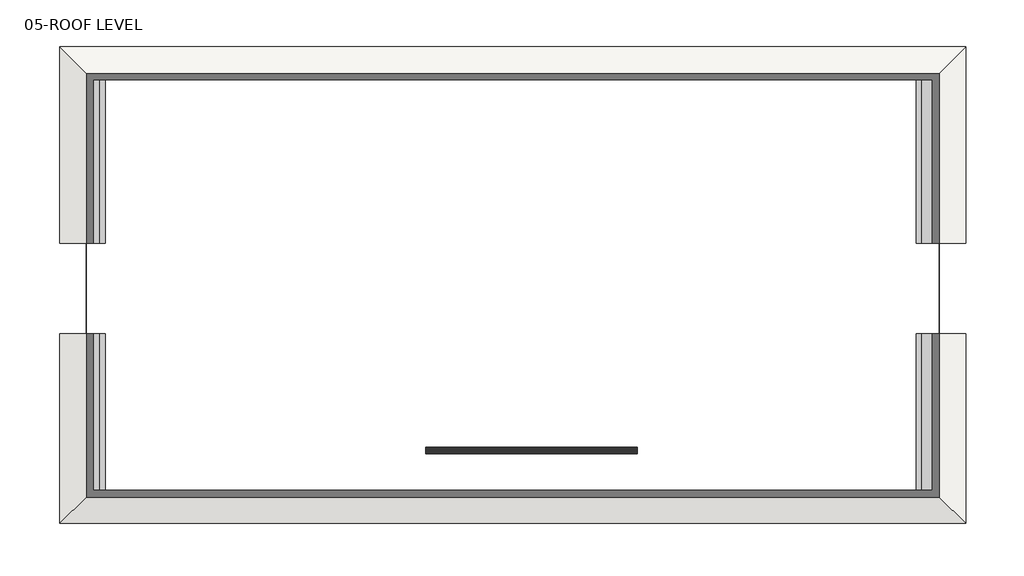
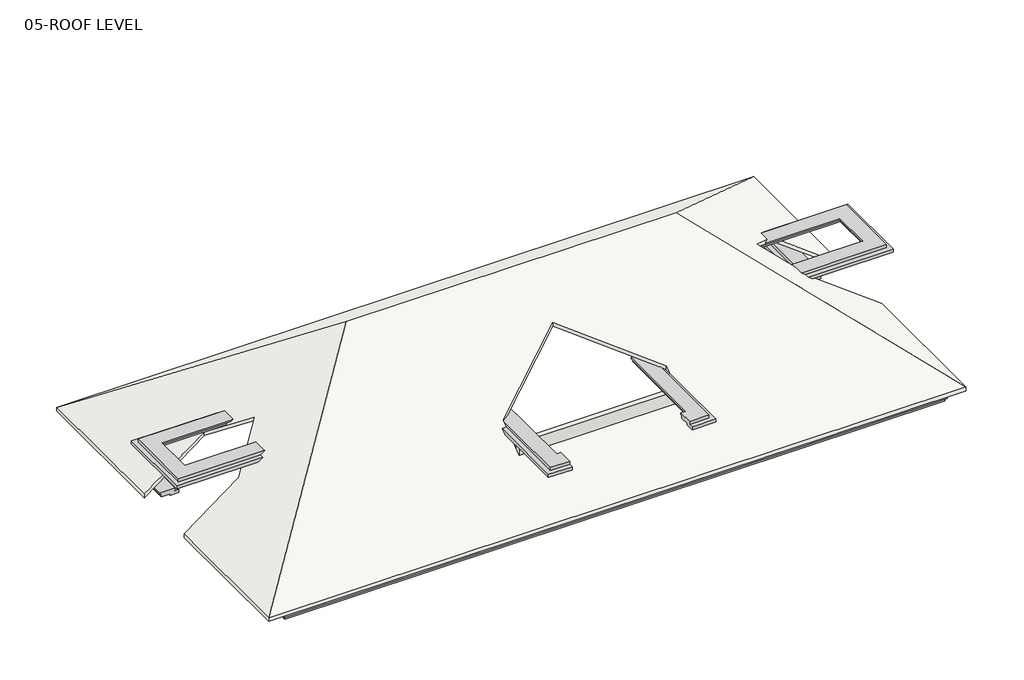
# One storey: 1 furniture element, 1 roof, 1 wall.
"""IFC4 building model written with IfcOpenShell, lengths in millimetres."""

from ifc_helpers import new_model, si_unit, origin, place, context, project, spatial, faceted_brep, transform, mapped, element, save
from components import casework_1_casework_1_4375437f

model = new_model("IFC4")

# Units and contexts
model_context = context("Model", 3, world=origin())
ifc_project = project(units=[si_unit("LENGTHUNIT", "METRE", prefix="MILLI")], contexts=[model_context])

# Site, building, storey
site = spatial("IfcSite", under=ifc_project)
building = spatial("IfcBuilding", under=site)
storey = spatial("IfcBuildingStorey", under=building, Name="05-ROOF LEVEL", Elevation=4500.0)

# Furniture
placement = place(None, origin())
casework_1_casework_1_shape = casework_1_casework_1_4375437f(model_context)
element("IfcFurniture", 1, ObjectType="Casework 1 : Casework 1", at=placement, inside=storey, context=model_context, shape_type="MappedRepresentation", body=[
    mapped(casework_1_casework_1_shape, transform((0.0, 0.0, 0.0), x_axis=(1.0, 0.0, 0.0), y_axis=(0.0, 1.0, 0.0), z_axis=(0.0, 0.0, 1.0))),
])

# Roof
element("IfcRoof", 2, ObjectType="01-roof sheet", at=placement, inside=storey, context=model_context, shape_type="Brep", body=[
    faceted_brep([(-8343.5169632, -3615.5592374, 6900.0), (-11143.5169632, -3615.5592374, 4800.0), (-11143.5169632, 3446.9407626, 4800.0), (-2581.0169632, -5115.5592374, 11221.875), (-11143.5169632, -13678.0592374, 4800.0), (-11143.5169632, -6865.5592374, 4800.0), (-8612.5649482, -6865.5592374, 6698.2140113), (-6853.0409557, -5106.0352449, 8017.8570056), (21381.0830368, -13678.0592374, 4800.0), (12818.5830368, -5115.5592374, 11221.875), (21381.0830368, 3446.9407626, 4800.0), (21381.0830368, -3615.5592374, 4800.0), (18128.5830368, -3615.5592374, 7239.375), (16503.5830368, -5240.5592374, 8458.125), (18128.5830368, -6865.5592374, 7239.375), (21381.0830368, -6865.5592374, 4800.0), (1993.5830368, -9865.5592374, 7659.375), (1993.5830368, -11165.5592374, 6684.375), (9593.5830368, -11165.5592374, 6684.375), (9593.5830368, -9865.5592374, 7659.375), (5793.5830368, -7302.4268734, 9581.724273), (-11143.5169632, -3615.5592374, 4987.5), (-8343.5169632, -3615.5592374, 7087.5), (-6853.0409557, -5106.0352449, 8205.3570056), (-8612.5649482, -6865.5592374, 6885.7140113), (-11143.5169632, -6865.5592374, 4987.5), (-11143.5169632, -13678.0592374, 4987.5), (-2581.0169632, -5115.5592374, 11409.375), (-11143.5169632, 3446.9407626, 4987.5), (21381.0830368, -13678.0592374, 4987.5), (21381.0830368, -6865.5592374, 4987.5), (18128.5830368, -6865.5592374, 7426.875), (16503.5830368, -5240.5592374, 8645.625), (18128.5830368, -3615.5592374, 7426.875), (21381.0830368, -3615.5592374, 4987.5), (21381.0830368, 3446.9407626, 4987.5), (12818.5830368, -5115.5592374, 11409.375), (1993.5830368, -11165.5592374, 6871.875), (1993.5830368, -9865.5592374, 7846.875), (5793.5830368, -7302.4268734, 9769.224273), (9593.5830368, -9865.5592374, 7846.875), (9593.5830368, -11165.5592374, 6871.875)], [[[0, 1, 2, 3, 4, 5, 6, 7]], [[8, 9, 10, 11, 12, 13, 14, 15]], [[3, 2, 10, 9]], [[4, 3, 9, 8], [16, 17, 18, 19, 20]], [[21, 22, 23, 24, 25, 26, 27, 28]], [[29, 30, 31, 32, 33, 34, 35, 36]], [[28, 27, 36, 35]], [[27, 26, 29, 36], [37, 38, 39, 40, 41]], [[26, 25, 5, 4]], [[29, 26, 4, 8]], [[30, 29, 8, 15]], [[35, 34, 11, 10]], [[28, 35, 10, 2]], [[21, 28, 2, 1]], [[12, 11, 34, 33]], [[15, 14, 31, 30]], [[13, 12, 33, 32]], [[14, 13, 32, 31]], [[1, 0, 22, 21]], [[6, 5, 25, 24]], [[0, 7, 23, 22]], [[7, 6, 24, 23]], [[37, 17, 16, 38]], [[40, 19, 18, 41]], [[17, 37, 41, 18]], [[38, 16, 20, 39]], [[19, 40, 39, 20]]]),
])

# Wall
element("IfcWall", 3, ObjectType="01-225 WALL", at=placement, inside=storey, context=model_context, shape_type="Brep", body=[
    faceted_brep([(1993.5830368, -11165.5592374, 4500.0), (9593.5830368, -11165.5592374, 4500.0), (9593.5830368, -11165.5592374, 7500.0), (1993.5830368, -11165.5592374, 7500.0), (1993.5830368, -10940.5592374, 4500.0), (1993.5830368, -10940.5592374, 7500.0), (2218.5830368, -10940.5592374, 7500.0), (9368.5830368, -10940.5592374, 7500.0), (9593.5830368, -10940.5592374, 7500.0), (9593.5830368, -10940.5592374, 4500.0)], [[[0, 1, 2, 3]], [[4, 5, 6, 7, 8, 9]], [[1, 0, 4, 9]], [[3, 2, 8, 7, 6, 5]], [[2, 1, 9, 8]], [[0, 3, 5, 4]]]),
])

save(model, "model.ifc")

# Revit data of these elements
# Type "01-roof sheet"
#   Description = "Generic Roof (Material By Category), 225mm thick"
#   Assembly Code = "B1020"
#   Type Mark = "G01"
#   Layers, outside or top first: 150 mm "roof" (function 1)
# Type "01-225 WALL"
#   Description = "Generic Wall (Material By Category), 200mm thick"
#   Assembly Code = "B2010"
#   Type Mark = "G06"
#   Layers, outside or top first: 225 mm "01-WHITE WALL" (function 1)
# Element 1 (IfcFurniture, "Casework 1 : Casework 1")
#   Phase Created = New Construction
# Element 2 (IfcRoof, "01-roof sheet")
#   built-in parameter 1001705 = 37.4323 (stored number, unit not read)
#   built-in parameter 1001701 = 0.984252 (stored number, unit not read)
#   built-in parameter 1001710 = 33615
#   Phase Created = New Construction
#   Materials on its faces: "roof"
# Element 3 (IfcWall, "01-225 WALL")
#   Top Offset = 0 mm
#   Base Offset = 0 mm
#   wall height = 3000 mm
#   Phase Created = New Construction
#   Base Constraint = 05-ROOF LEVEL
#   Materials on its faces: "01-WHITE WALL"
# Materials
#   "roof": class "Generic", colour RGB 120 120 120, transparency 0, Cost = 0
#   "01-WHITE WALL": class "Generic", colour RGB 244 244 244, transparency 0, Description = "Acoustic Ceiling Tile 24 x 48", Cost = 0
